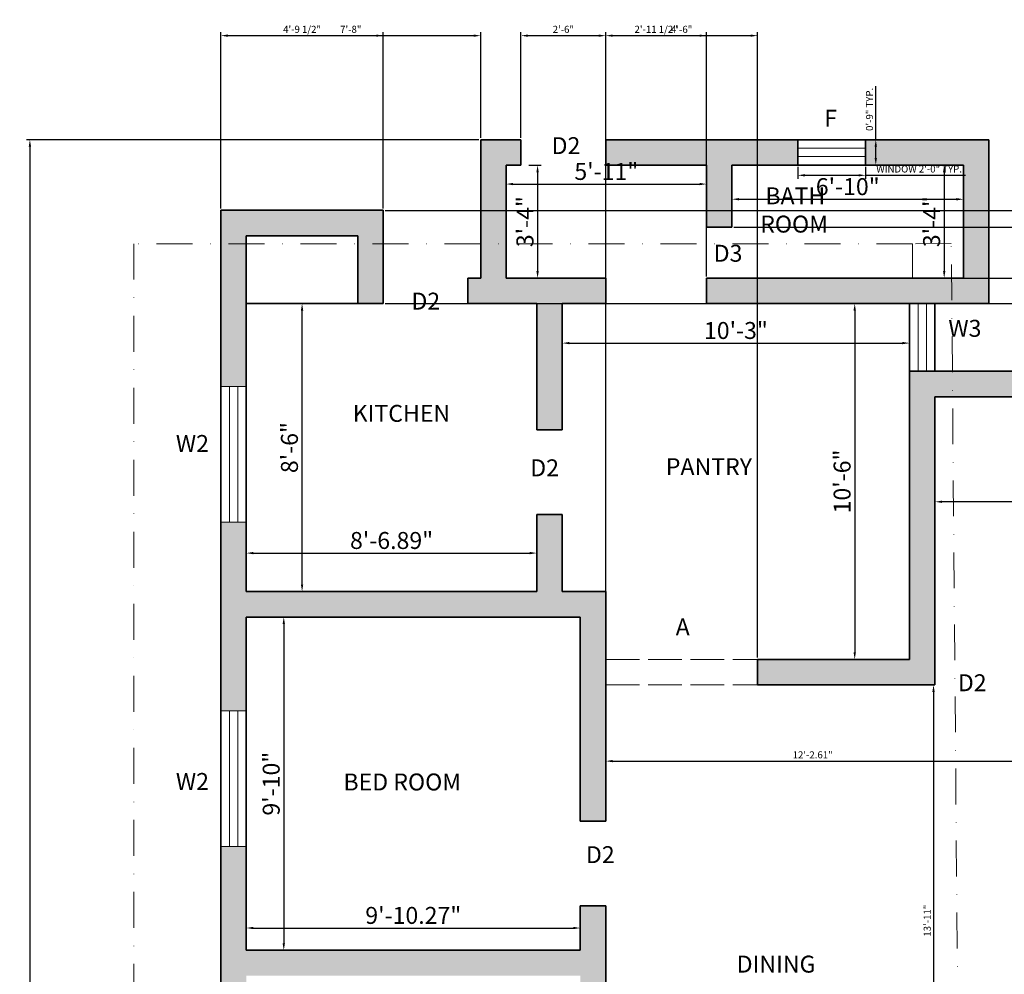
# Model space of a CAD drawing. Units: inches. Extents: x 4701 to 5398, y 2331 to 3130.
# Tile 2 of 3: x 4701 to 5050, y 2792 to 3130. Entities that reach past the tile are written whole.
import ezdxf

# ---------------------------------------------------------------- set-up
doc = ezdxf.new("R2010")
doc.units = ezdxf.units.IN
doc.linetypes.add('ACAD_ISO02W100', pattern=[15, 12, -3])
doc.linetypes.add('DASHDOT', pattern=[25.4, 12.7, -6.35, 0, -6.35])
for name, color, linetype, lineweight, true_color in [('A-ANNO-DIMS', 217, 'Continuous', 18, 0x93278f), ('A-GLAZ', 41, 'Continuous', 18, 0xf4ee51), ('A-WALL-OVHD', 41, 'ACAD_ISO02W100', 18, 0xf4ee51), ('A-WALL-PATT', 143, 'Continuous', 13, 0x7aafdf)]:
    doc.layers.add(name, color=color, linetype=linetype, lineweight=lineweight, true_color=true_color)
for name, color, linetype, lineweight in [('A-ANNO-TEXT', 7, 'Continuous', 18), ('A-AREA-IDEN', 7, 'Continuous', 25), ('A-ROOF-OVHD', 8, 'DASHDOT', 13), ('A-WALL', 7, 'Continuous', 35)]:
    doc.layers.add(name, color=color, linetype=linetype, lineweight=lineweight)
doc.styles.get("Standard").update_dxf_attribs({"font": 'arial.ttf'})
doc.dimstyles.new('ISO-25', dxfattribs={"dimtxt": 2.5, "dimasz": 2.5, "dimexe": 1.25, "dimexo": 0.625, "dimtad": 1, "dimlunit": 3, "dimtxsty": 'Standard', "dimcen": 2.5, "dimadec": 0, "dimazin": 0, "dimtfac": 1, "dimtmove": 0, "dimatfit": 3, "dimfxl": 1, "dimarcsym": 0})

# ---------------------------------------------------------------- blocks, each defined once
blk = doc.blocks.new('*D1')
at = {"layer": 'A-ANNO-DIMS', "color": 0, "lineweight": -2, "transparency": 16777216}
for p, q in [((4873.22, 3071.97), (4873.22, 3072.6)), ((4944.22, 3071.97), (4944.22, 3072.6)), ((4875.72, 3071.35), (4941.72, 3071.35))]:
    blk.add_line(p, q, dxfattribs=at)
at = {"layer": 'A-ANNO-DIMS', "color": 0, "transparency": 16777216}
for points in [[(4875.72, 3071.77), (4875.72, 3070.93), (4873.22, 3071.35)], [(4941.72, 3071.77), (4941.72, 3070.93), (4944.22, 3071.35)]]:
    blk.add_solid(points, dxfattribs=at)
at = {"layer": 'Defpoints', "color": 0, "transparency": 16777216}
for p in [(4873.22, 3071.35), (4944.22, 3071.35), (4944.22, 3071.35)]:
    blk.add_point(p, dxfattribs=at)
at = {"layer": 'A-ANNO-DIMS', "color": 0, "transparency": 16777216, "insert": (4908.72, 3075.04), "char_height": 6, "attachment_point": 5}
blk.add_mtext('5\'-11"', dxfattribs=at)
blk = doc.blocks.new('*D2')
at = {"layer": 'A-ANNO-DIMS', "color": 0, "lineweight": -2, "transparency": 16777216}
for p, q in [((4953.22, 3066.43), (4953.22, 3064.73)), ((4955.72, 3065.98), (5032.72, 3065.98)), ((5035.22, 3066.61), (5035.22, 3067.23))]:
    blk.add_line(p, q, dxfattribs=at)
at = {"layer": 'A-ANNO-DIMS', "color": 0, "transparency": 16777216}
for points in [[(4955.72, 3066.4), (4955.72, 3065.57), (4953.22, 3065.98)], [(5032.72, 3066.4), (5032.72, 3065.57), (5035.22, 3065.98)]]:
    blk.add_solid(points, dxfattribs=at)
at = {"layer": 'Defpoints', "color": 0, "transparency": 16777216}
for p in [(4953.22, 3067.05), (5035.22, 3065.98), (5035.22, 3065.98)]:
    blk.add_point(p, dxfattribs=at)
at = {"layer": 'A-ANNO-DIMS', "color": 0, "transparency": 16777216, "insert": (4994.22, 3069.67), "char_height": 6, "attachment_point": 5}
blk.add_mtext('6\'-10"', dxfattribs=at)
blk = doc.blocks.new('*D3')
at = {"layer": 'A-ANNO-DIMS', "color": 0, "lineweight": -2, "transparency": 16777216}
for p, q in [((4881.25, 3078.05), (4885.63, 3078.05)), ((4884.38, 3075.55), (4884.38, 3040.55)), ((4881.25, 3038.05), (4885.63, 3038.05))]:
    blk.add_line(p, q, dxfattribs=at)
at = {"layer": 'A-ANNO-DIMS', "color": 0, "transparency": 16777216}
for points in [[(4883.96, 3075.55), (4884.8, 3075.55), (4884.38, 3078.05)], [(4883.96, 3040.55), (4884.8, 3040.55), (4884.38, 3038.05)]]:
    blk.add_solid(points, dxfattribs=at)
at = {"layer": 'Defpoints', "color": 0, "transparency": 16777216}
for p in [(4880.63, 3078.05), (4880.63, 3038.05), (4884.38, 3038.05)]:
    blk.add_point(p, dxfattribs=at)
at = {"layer": 'A-ANNO-DIMS', "color": 0, "transparency": 16777216, "insert": (4880.69, 3058.05), "char_height": 6, "attachment_point": 5, "rotation": 90}
blk.add_mtext('3\'-4"', dxfattribs=at)
blk = doc.blocks.new('*D4')
at = {"layer": 'A-ANNO-DIMS', "color": 0, "lineweight": -2, "transparency": 16777216}
for p, q in [((5027.76, 3078.05), (5027.13, 3078.05)), ((5028.38, 3075.55), (5028.38, 3040.55)), ((5027.76, 3038.05), (5027.13, 3038.05))]:
    blk.add_line(p, q, dxfattribs=at)
at = {"layer": 'A-ANNO-DIMS', "color": 0, "transparency": 16777216}
for points in [[(5027.97, 3075.55), (5028.8, 3075.55), (5028.38, 3078.05)], [(5027.97, 3040.55), (5028.8, 3040.55), (5028.38, 3038.05)]]:
    blk.add_solid(points, dxfattribs=at)
at = {"layer": 'Defpoints', "color": 0, "transparency": 16777216}
for p in [(5028.38, 3078.05), (5028.38, 3038.05), (5028.38, 3038.05)]:
    blk.add_point(p, dxfattribs=at)
at = {"layer": 'A-ANNO-DIMS', "color": 0, "transparency": 16777216, "insert": (5024.69, 3058.05), "char_height": 6, "attachment_point": 5, "rotation": 90}
blk.add_mtext('3\'-4"', dxfattribs=at)
blk = doc.blocks.new('*D5')
at = {"layer": 'A-ANNO-DIMS', "color": 0, "lineweight": -2, "transparency": 16777216}
for p, q in [((4801.6, 3029.05), (4802.22, 3029.05)), ((4800.97, 2929.55), (4800.97, 3026.55)), ((4801.6, 2927.05), (4799.72, 2927.05))]:
    blk.add_line(p, q, dxfattribs=at)
at = {"layer": 'A-ANNO-DIMS', "color": 0, "transparency": 16777216}
for points in [[(4800.56, 3026.55), (4801.39, 3026.55), (4800.97, 3029.05)], [(4800.56, 2929.55), (4801.39, 2929.55), (4800.97, 2927.05)]]:
    blk.add_solid(points, dxfattribs=at)
at = {"layer": 'Defpoints', "color": 0, "transparency": 16777216}
for p in [(4800.97, 3029.05), (4800.97, 3029.05), (4802.22, 2927.05)]:
    blk.add_point(p, dxfattribs=at)
at = {"layer": 'A-ANNO-DIMS', "color": 0, "transparency": 16777216, "insert": (4797.28, 2978.05), "char_height": 6, "attachment_point": 5, "rotation": 90}
blk.add_mtext('8\'-6"', dxfattribs=at)
blk = doc.blocks.new('*D6')
at = {"layer": 'A-ANNO-DIMS', "color": 0, "lineweight": -2, "transparency": 16777216}
for p, q in [((4781.22, 2941.32), (4781.22, 2941.94)), ((4783.72, 2940.69), (4881.61, 2940.69)), ((4884.11, 2941.32), (4884.11, 2941.94))]:
    blk.add_line(p, q, dxfattribs=at)
at = {"layer": 'A-ANNO-DIMS', "color": 0, "transparency": 16777216}
for points in [[(4783.72, 2941.11), (4783.72, 2940.27), (4781.22, 2940.69)], [(4881.61, 2941.11), (4881.61, 2940.27), (4884.11, 2940.69)]]:
    blk.add_solid(points, dxfattribs=at)
at = {"layer": 'Defpoints', "color": 0, "transparency": 16777216}
for p in [(4781.22, 2940.69), (4884.11, 2940.69), (4884.11, 2940.69)]:
    blk.add_point(p, dxfattribs=at)
at = {"layer": 'A-ANNO-DIMS', "color": 0, "transparency": 16777216, "insert": (4832.67, 2944.38), "char_height": 6, "attachment_point": 5}
blk.add_mtext('8\'-6.89"', dxfattribs=at)
blk = doc.blocks.new('*D7')
at = {"layer": 'A-ANNO-DIMS', "color": 0, "lineweight": -2, "transparency": 16777216}
for p, q in [((4893.11, 3015.67), (4893.11, 3016.29)), ((5016.11, 3015.67), (5016.11, 3016.29)), ((4895.61, 3015.04), (5013.61, 3015.04))]:
    blk.add_line(p, q, dxfattribs=at)
at = {"layer": 'A-ANNO-DIMS', "color": 0, "transparency": 16777216}
for points in [[(4895.61, 3015.46), (4895.61, 3014.63), (4893.11, 3015.04)], [(5013.61, 3015.46), (5013.61, 3014.63), (5016.11, 3015.04)]]:
    blk.add_solid(points, dxfattribs=at)
at = {"layer": 'Defpoints', "color": 0, "transparency": 16777216}
for p in [(4893.11, 3015.04), (5016.11, 3015.04), (5016.11, 3015.04)]:
    blk.add_point(p, dxfattribs=at)
at = {"layer": 'A-ANNO-DIMS', "color": 0, "transparency": 16777216, "insert": (4954.61, 3018.73), "char_height": 6, "attachment_point": 5}
blk.add_mtext('10\'-3"', dxfattribs=at)
blk = doc.blocks.new('*D8')
at = {"layer": 'A-ANNO-DIMS', "color": 0, "lineweight": -2, "transparency": 16777216}
for p, q in [((4999.81, 3029.05), (4995.44, 3029.05)), ((4996.69, 3026.55), (4996.69, 2905.55)), ((4997.31, 2903.05), (4997.94, 2903.05))]:
    blk.add_line(p, q, dxfattribs=at)
at = {"layer": 'A-ANNO-DIMS', "color": 0, "transparency": 16777216}
for points in [[(4996.27, 3026.55), (4997.11, 3026.55), (4996.69, 3029.05)], [(4996.27, 2905.55), (4997.11, 2905.55), (4996.69, 2903.05)]]:
    blk.add_solid(points, dxfattribs=at)
at = {"layer": 'Defpoints', "color": 0, "transparency": 16777216}
for p in [(5000.44, 3029.05), (4996.69, 2903.05), (4996.69, 2903.05)]:
    blk.add_point(p, dxfattribs=at)
at = {"layer": 'A-ANNO-DIMS', "color": 0, "transparency": 16777216, "insert": (4993, 2966.05), "char_height": 6, "attachment_point": 5, "rotation": 90}
blk.add_mtext('10\'-6"', dxfattribs=at)
blk = doc.blocks.new('*D9')
at = {"layer": 'A-ANNO-DIMS', "color": 0, "lineweight": -2, "transparency": 16777216}
for p, q in [((5025.11, 2959.48), (5025.11, 2960.11)), ((5190.61, 2958.86), (5027.61, 2958.86)), ((5193.11, 2959.48), (5193.11, 2960.11))]:
    blk.add_line(p, q, dxfattribs=at)
at = {"layer": 'A-ANNO-DIMS', "color": 0, "transparency": 16777216}
for points in [[(5027.61, 2959.28), (5027.61, 2958.44), (5025.11, 2958.86)], [(5190.61, 2959.28), (5190.61, 2958.44), (5193.11, 2958.86)]]:
    blk.add_solid(points, dxfattribs=at)
at = {"layer": 'Defpoints', "color": 0, "transparency": 16777216}
for p in [(5025.11, 2958.86), (5025.11, 2958.86), (5193.11, 2958.86)]:
    blk.add_point(p, dxfattribs=at)
at = {"layer": 'A-ANNO-DIMS', "color": 0, "transparency": 16777216, "insert": (5109.11, 2962.5), "char_height": 6, "attachment_point": 5}
blk.add_mtext("14'", dxfattribs=at)
blk = doc.blocks.new('*D13')
at = {"layer": 'A-ANNO-DIMS', "color": 0, "lineweight": -2, "transparency": 16777216}
for p, q in [((4781.22, 2808.57), (4781.22, 2809.19)), ((4783.72, 2807.94), (4897, 2807.94)), ((4899.5, 2808.57), (4899.5, 2809.19))]:
    blk.add_line(p, q, dxfattribs=at)
at = {"layer": 'A-ANNO-DIMS', "color": 0, "transparency": 16777216}
for points in [[(4783.72, 2808.36), (4783.72, 2807.53), (4781.22, 2807.94)], [(4897, 2808.36), (4897, 2807.53), (4899.5, 2807.94)]]:
    blk.add_solid(points, dxfattribs=at)
at = {"layer": 'Defpoints', "color": 0, "transparency": 16777216}
for p in [(4781.22, 2807.94), (4899.5, 2807.94), (4899.5, 2807.94)]:
    blk.add_point(p, dxfattribs=at)
at = {"layer": 'A-ANNO-DIMS', "color": 0, "transparency": 16777216, "insert": (4840.36, 2811.63), "char_height": 6, "attachment_point": 5}
blk.add_mtext('9\'-10.27"', dxfattribs=at)
blk = doc.blocks.new('*D14')
at = {"layer": 'A-ANNO-DIMS', "color": 0, "lineweight": -2, "transparency": 16777216}
for p, q in [((4794.49, 2915.55), (4794.49, 2802.55)), ((4795.12, 2918.05), (4795.74, 2918.05)), ((4795.12, 2800.05), (4795.74, 2800.05))]:
    blk.add_line(p, q, dxfattribs=at)
at = {"layer": 'A-ANNO-DIMS', "color": 0, "transparency": 16777216}
for points in [[(4794.08, 2915.55), (4794.91, 2915.55), (4794.49, 2918.05)], [(4794.08, 2802.55), (4794.91, 2802.55), (4794.49, 2800.05)]]:
    blk.add_solid(points, dxfattribs=at)
at = {"layer": 'Defpoints', "color": 0, "transparency": 16777216}
for p in [(4794.49, 2918.05), (4794.49, 2800.05), (4794.49, 2800.05)]:
    blk.add_point(p, dxfattribs=at)
at = {"layer": 'A-ANNO-DIMS', "color": 0, "transparency": 16777216, "insert": (4790.81, 2859.05), "char_height": 6, "attachment_point": 5, "rotation": 90}
blk.add_mtext('9\'-10"', dxfattribs=at)
blk = doc.blocks.new('*D29')
at = {"layer": 'A-ANNO-DIMS', "color": 0, "lineweight": -2, "transparency": 16777216}
for p, q in [((4908.5, 2867.66), (4908.5, 2868.28)), ((4911, 2867.03), (5052.61, 2867.03)), ((5055.11, 2867.66), (5055.11, 2868.28))]:
    blk.add_line(p, q, dxfattribs=at)
at = {"layer": 'A-ANNO-DIMS', "color": 0, "transparency": 16777216}
for points in [[(4911, 2867.45), (4911, 2866.62), (4908.5, 2867.03)], [(5052.61, 2867.45), (5052.61, 2866.62), (5055.11, 2867.03)]]:
    blk.add_solid(points, dxfattribs=at)
at = {"layer": 'Defpoints', "color": 0, "transparency": 16777216}
for p in [(4908.5, 2867.03), (5055.11, 2867.03), (5055.11, 2867.03)]:
    blk.add_point(p, dxfattribs=at)
at = {"layer": 'A-ANNO-DIMS', "color": 0, "transparency": 16777216, "insert": (4981.8, 2868.94), "char_height": 2.5, "attachment_point": 5}
blk.add_mtext('12\'-2.61"', dxfattribs=at)
blk = doc.blocks.new('*D30')
at = {"layer": 'A-ANNO-DIMS', "color": 0, "lineweight": -2, "transparency": 16777216}
for p, q in [((5024.48, 2894.05), (5023.35, 2894.05)), ((5024.6, 2891.55), (5024.6, 2729.55)), ((5025.23, 2727.05), (5025.85, 2727.05))]:
    blk.add_line(p, q, dxfattribs=at)
at = {"layer": 'A-ANNO-DIMS', "color": 0, "transparency": 16777216}
for points in [[(5024.19, 2891.55), (5025.02, 2891.55), (5024.6, 2894.05)], [(5024.19, 2729.55), (5025.02, 2729.55), (5024.6, 2727.05)]]:
    blk.add_solid(points, dxfattribs=at)
at = {"layer": 'Defpoints', "color": 0, "transparency": 16777216}
for p in [(5025.11, 2894.05), (5024.6, 2727.05), (5024.6, 2727.05)]:
    blk.add_point(p, dxfattribs=at)
at = {"layer": 'A-ANNO-DIMS', "color": 0, "transparency": 16777216, "insert": (5022.7, 2810.55), "char_height": 2.5, "attachment_point": 5, "rotation": 90}
blk.add_mtext('13\'-11"', dxfattribs=at)
blk = doc.blocks.new('WIN-48IN')
for p, q in [((0, 48), (9, 48)), ((0, 48), (0, 0)), ((3, 48), (3, 0)), ((6, 48), (6, 0)), ((9, 0), (9, 48)), ((0, 0), (9, 0))]:
    blk.add_line(p, q)
blk = doc.blocks.new('WIN-24IN')
for p, q in [((0, 9), (0, 0)), ((24, 9), (0, 9)), ((24, 0), (24, 9)), ((24, 6), (0, 6)), ((24, 3), (0, 3)), ((0, 0), (24, 0))]:
    blk.add_line(p, q)
blk = doc.blocks.new('*D39')
at = {"layer": 'A-ANNO-DIMS', "color": 0, "lineweight": -2, "transparency": 16777216}
for p, q in [((4976.55, 3077.43), (4976.55, 3073.2)), ((5000.55, 3077.43), (5000.55, 3073.2)), ((4979.05, 3074.45), (4998.05, 3074.45)), ((5000.55, 3074.45), (5035.93, 3074.45))]:
    blk.add_line(p, q, dxfattribs=at)
at = {"layer": 'A-ANNO-DIMS', "color": 0, "transparency": 16777216}
for points in [[(4979.05, 3074.87), (4979.05, 3074.04), (4976.55, 3074.45)], [(4998.05, 3074.87), (4998.05, 3074.04), (5000.55, 3074.45)]]:
    blk.add_solid(points, dxfattribs=at)
at = {"layer": 'Defpoints', "color": 0, "transparency": 16777216}
for p in [(4976.55, 3078.05), (5000.55, 3078.05), (5000.55, 3074.45)]:
    blk.add_point(p, dxfattribs=at)
at = {"layer": 'A-ANNO-DIMS', "color": 0, "transparency": 16777216, "insert": (5019.49, 3076.37), "char_height": 2.5, "attachment_point": 5}
blk.add_mtext('WINDOW 2\'-0" TYP.', dxfattribs=at)
blk = doc.blocks.new('*D40')
at = {"layer": 'A-ANNO-DIMS', "color": 0, "lineweight": -2, "transparency": 16777216}
for p, q in [((5004.15, 3087.05), (5004.15, 3106.04)), ((5001.17, 3087.05), (5005.4, 3087.05)), ((5004.15, 3080.55), (5004.15, 3084.55)), ((5001.17, 3078.05), (5005.4, 3078.05))]:
    blk.add_line(p, q, dxfattribs=at)
at = {"layer": 'A-ANNO-DIMS', "color": 0, "transparency": 16777216}
for points in [[(5003.73, 3084.55), (5004.56, 3084.55), (5004.15, 3087.05)], [(5003.73, 3080.55), (5004.56, 3080.55), (5004.15, 3078.05)]]:
    blk.add_solid(points, dxfattribs=at)
at = {"layer": 'Defpoints', "color": 0, "transparency": 16777216}
for p in [(5000.55, 3087.05), (5004.15, 3087.05), (5000.55, 3078.05)]:
    blk.add_point(p, dxfattribs=at)
at = {"layer": 'A-ANNO-DIMS', "color": 0, "transparency": 16777216, "insert": (5002.24, 3097.8), "char_height": 2.5, "attachment_point": 5, "rotation": 90}
blk.add_mtext('0\'-9" TYP.', dxfattribs=at)
blk = doc.blocks.new('*D44')
at = {"layer": 'A-ANNO-DIMS', "color": 0, "lineweight": -2, "transparency": 16777216}
for p, q in [((4863.6, 3087.05), (4703.32, 3087.05)), ((4704.57, 3084.55), (4704.57, 2407.55)), ((4985.68, 2405.05), (4703.32, 2405.05))]:
    blk.add_line(p, q, dxfattribs=at)
at = {"layer": 'A-ANNO-DIMS', "color": 0, "transparency": 16777216}
for points in [[(4704.15, 3084.55), (4704.99, 3084.55), (4704.57, 3087.05)], [(4704.15, 2407.55), (4704.99, 2407.55), (4704.57, 2405.05)]]:
    blk.add_solid(points, dxfattribs=at)
at = {"layer": 'Defpoints', "color": 0, "transparency": 16777216}
for p in [(4864.22, 3087.05), (4704.57, 2405.05), (4986.3, 2405.05)]:
    blk.add_point(p, dxfattribs=at)
at = {"layer": 'A-ANNO-DIMS', "color": 0, "transparency": 16777216, "insert": (4702.67, 2746.05), "char_height": 2.5, "attachment_point": 5, "rotation": 90}
blk.add_mtext('56\'-10"', dxfattribs=at)
blk = doc.blocks.new('*D46')
at = {"layer": 'A-ANNO-DIMS', "color": 0, "lineweight": -2, "transparency": 16777216}
for p, q in [((4878.5, 3087.68), (4878.5, 3125.15)), ((4908.5, 3087.68), (4908.5, 3125.15)), ((4881, 3123.9), (4906, 3123.9))]:
    blk.add_line(p, q, dxfattribs=at)
at = {"layer": 'A-ANNO-DIMS', "color": 0, "transparency": 16777216}
for points in [[(4881, 3124.32), (4881, 3123.49), (4878.5, 3123.9)], [(4906, 3124.32), (4906, 3123.49), (4908.5, 3123.9)]]:
    blk.add_solid(points, dxfattribs=at)
at = {"layer": 'Defpoints', "color": 0, "transparency": 16777216}
for p in [(4908.5, 3123.9), (4878.5, 3087.05), (4908.5, 3087.05)]:
    blk.add_point(p, dxfattribs=at)
at = {"layer": 'A-ANNO-DIMS', "color": 0, "transparency": 16777216, "insert": (4893.5, 3125.81), "char_height": 2.5, "attachment_point": 5}
blk.add_mtext('2\'-6"', dxfattribs=at)
blk = doc.blocks.new('*D47')
at = {"layer": 'A-ANNO-DIMS', "color": 0, "lineweight": -2, "transparency": 16777216}
for p, q in [((4908.5, 3038.68), (4908.5, 3125.15)), ((4944.22, 3038.68), (4944.22, 3125.15)), ((4911, 3123.9), (4941.72, 3123.9))]:
    blk.add_line(p, q, dxfattribs=at)
at = {"layer": 'A-ANNO-DIMS', "color": 0, "transparency": 16777216}
for points in [[(4911, 3124.32), (4911, 3123.49), (4908.5, 3123.9)], [(4941.72, 3124.32), (4941.72, 3123.49), (4944.22, 3123.9)]]:
    blk.add_solid(points, dxfattribs=at)
at = {"layer": 'Defpoints', "color": 0, "transparency": 16777216}
for p in [(4944.22, 3123.9), (4908.5, 3038.05), (4944.22, 3038.05)]:
    blk.add_point(p, dxfattribs=at)
at = {"layer": 'A-ANNO-DIMS', "color": 0, "transparency": 16777216, "insert": (4926.36, 3125.82), "char_height": 2.5, "attachment_point": 5}
blk.add_mtext('2\'-11 1/2"', dxfattribs=at)
blk = doc.blocks.new('*D49')
at = {"layer": 'A-ANNO-DIMS', "color": 0, "lineweight": -2, "transparency": 16777216}
for p, q in [((4908.5, 2903.68), (4908.5, 3125.15)), ((4962.3, 2903.68), (4962.3, 3125.15)), ((4911, 3123.9), (4959.8, 3123.9))]:
    blk.add_line(p, q, dxfattribs=at)
at = {"layer": 'A-ANNO-DIMS', "color": 0, "transparency": 16777216}
for points in [[(4911, 3124.32), (4911, 3123.49), (4908.5, 3123.9)], [(4959.8, 3124.32), (4959.8, 3123.49), (4962.3, 3123.9)]]:
    blk.add_solid(points, dxfattribs=at)
at = {"layer": 'Defpoints', "color": 0, "transparency": 16777216}
for p in [(4962.3, 3123.9), (4908.5, 2903.05), (4962.3, 2903.05)]:
    blk.add_point(p, dxfattribs=at)
at = {"layer": 'A-ANNO-DIMS', "color": 0, "transparency": 16777216, "insert": (4935.4, 3125.81), "char_height": 2.5, "attachment_point": 5}
blk.add_mtext('4\'-6"', dxfattribs=at)
blk = doc.blocks.new('*D51')
at = {"layer": 'A-ANNO-DIMS', "color": 0, "lineweight": -2, "transparency": 16777216}
for p, q in [((4772.22, 3062.68), (4772.22, 3125.15)), ((4864.22, 3087.68), (4864.22, 3125.15)), ((4774.72, 3123.9), (4861.72, 3123.9))]:
    blk.add_line(p, q, dxfattribs=at)
at = {"layer": 'A-ANNO-DIMS', "color": 0, "transparency": 16777216}
for points in [[(4774.72, 3124.32), (4774.72, 3123.49), (4772.22, 3123.9)], [(4861.72, 3124.32), (4861.72, 3123.49), (4864.22, 3123.9)]]:
    blk.add_solid(points, dxfattribs=at)
at = {"layer": 'Defpoints', "color": 0, "transparency": 16777216}
for p in [(4864.22, 3123.9), (4864.22, 3087.05), (4772.22, 3062.05)]:
    blk.add_point(p, dxfattribs=at)
at = {"layer": 'A-ANNO-DIMS', "color": 0, "transparency": 16777216, "insert": (4818.22, 3125.81), "char_height": 2.5, "attachment_point": 5}
blk.add_mtext('7\'-8"', dxfattribs=at)
blk = doc.blocks.new('*D52')
at = {"layer": 'A-ANNO-DIMS', "color": 0, "lineweight": -2, "transparency": 16777216}
for p, q in [((4772.22, 3062.68), (4772.22, 3125.15)), ((4829.72, 3062.68), (4829.72, 3125.15)), ((4774.72, 3123.9), (4827.22, 3123.9))]:
    blk.add_line(p, q, dxfattribs=at)
at = {"layer": 'A-ANNO-DIMS', "color": 0, "transparency": 16777216}
for points in [[(4774.72, 3124.32), (4774.72, 3123.49), (4772.22, 3123.9)], [(4827.22, 3124.32), (4827.22, 3123.49), (4829.72, 3123.9)]]:
    blk.add_solid(points, dxfattribs=at)
at = {"layer": 'Defpoints', "color": 0, "transparency": 16777216}
for p in [(4829.72, 3123.9), (4772.22, 3062.05), (4829.72, 3062.05)]:
    blk.add_point(p, dxfattribs=at)
at = {"layer": 'A-ANNO-DIMS', "color": 0, "transparency": 16777216, "insert": (4800.97, 3125.82), "char_height": 2.5, "attachment_point": 5}
blk.add_mtext('4\'-9 1/2"', dxfattribs=at)
blk = doc.blocks.new('*D53')
at = {"layer": 'A-ANNO-DIMS', "color": 0, "lineweight": -2, "transparency": 16777216}
for p, q in [((4830.35, 3062.05), (5398.37, 3062.05)), ((5397.12, 3059.55), (5397.12, 3031.55)), ((4830.35, 3029.05), (5398.37, 3029.05))]:
    blk.add_line(p, q, dxfattribs=at)
at = {"layer": 'A-ANNO-DIMS', "color": 0, "transparency": 16777216}
for points in [[(5396.71, 3059.55), (5397.54, 3059.55), (5397.12, 3062.05)], [(5396.71, 3031.55), (5397.54, 3031.55), (5397.12, 3029.05)]]:
    blk.add_solid(points, dxfattribs=at)
at = {"layer": 'Defpoints', "color": 0, "transparency": 16777216}
for p in [(4829.72, 3062.05), (4829.72, 3029.05), (5397.12, 3029.05)]:
    blk.add_point(p, dxfattribs=at)
at = {"layer": 'A-ANNO-DIMS', "color": 0, "transparency": 16777216, "insert": (5395.22, 3045.55), "char_height": 2.5, "attachment_point": 5, "rotation": 90}
blk.add_mtext('2\'-9"', dxfattribs=at)
blk = doc.blocks.new('*D54')
at = {"layer": 'A-ANNO-DIMS', "color": 0, "lineweight": -2, "transparency": 16777216}
for p, q in [((4953.85, 3056.05), (5398.37, 3056.05)), ((5397.12, 3053.55), (5397.12, 3040.55)), ((4944.85, 3038.05), (5398.37, 3038.05))]:
    blk.add_line(p, q, dxfattribs=at)
at = {"layer": 'A-ANNO-DIMS', "color": 0, "transparency": 16777216}
for points in [[(5396.71, 3053.55), (5397.54, 3053.55), (5397.12, 3056.05)], [(5396.71, 3040.55), (5397.54, 3040.55), (5397.12, 3038.05)]]:
    blk.add_solid(points, dxfattribs=at)
at = {"layer": 'Defpoints', "color": 0, "transparency": 16777216}
for p in [(4953.22, 3056.05), (4944.22, 3038.05), (5397.12, 3038.05)]:
    blk.add_point(p, dxfattribs=at)
at = {"layer": 'A-ANNO-DIMS', "color": 0, "transparency": 16777216, "insert": (5395.22, 3047.05), "char_height": 2.5, "attachment_point": 5, "rotation": 90}
blk.add_mtext('1\'-6"', dxfattribs=at)

msp = doc.modelspace()

# ---------------------------------------------------------------- hatches: boundary and pattern name
at = {"layer": 'A-WALL-PATT'}
h = msp.add_hatch(color=256, dxfattribs=at)
h.dxf.hatch_style = 1
h.paths.add_polyline_path([(4829.723, 3062.054), (4820.723, 3062.054), (4772.223, 3062.054), (4772.223, 3050.208), (4781.223, 3050.208), (4781.223, 3053.054), (4820.723, 3053.054), (4820.723, 3050.208), (4829.723, 3050.208)])
h.paths.add_polyline_path([(4781.223, 3050.208), (4772.223, 3050.208), (4772.223, 3029.054), (4772.223, 2999.675), (4781.223, 2999.675), (4781.223, 3029.054)])
h.paths.add_polyline_path([(4781.223, 2918.054), (4864.223, 2918.054), (4899.497, 2918.054), (4899.497, 2845.832), (4908.497, 2845.832), (4908.497, 2918.054), (4908.497, 2927.054), (4893.11, 2927.054), (4893.11, 2954.328), (4884.11, 2954.328), (4884.11, 2927.054), (4864.223, 2927.054), (4781.223, 2927.054), (4781.223, 2951.675), (4772.223, 2951.675), (4772.223, 2918.054), (4772.223, 2884.79), (4781.223, 2884.79)])
h.paths.add_polyline_path([(4893.11, 3029.054), (4908.497, 3029.054), (4908.497, 3038.054), (4873.223, 3038.054), (4873.223, 3050.208), (4864.223, 3050.208), (4864.223, 3038.054), (4859.723, 3038.054), (4859.723, 3029.054), (4884.11, 3029.054), (4884.11, 2984.328), (4893.11, 2984.328)])
h.paths.add_polyline_path([(4873.223, 3078.054), (4878.497, 3078.054), (4878.497, 3087.054), (4864.223, 3087.054), (4864.223, 3050.208), (4873.223, 3050.208)])
h.paths.add_polyline_path([(4976.546, 3087.054), (4908.497, 3087.054), (4908.497, 3078.054), (4944.223, 3078.054), (4944.223, 3056.054), (4953.223, 3056.054), (4953.223, 3078.054), (4976.546, 3078.054)])
h.paths.add_polyline_path([(5044.223, 3087.054), (5000.546, 3087.054), (5000.546, 3078.054), (5035.223, 3078.054), (5035.223, 3038.054), (5044.223, 3038.054)])
h.paths.add_polyline_path([(5030.994, 3038.054), (5017.16, 3038.054), (4944.223, 3038.054), (4944.223, 3029.054), (5031.069, 3029.054)])
h.paths.add_polyline_path([(5044.223, 3038.054), (5035.223, 3038.054), (5030.994, 3038.054), (5031.069, 3029.054), (5044.223, 3029.054)])
h.paths.add_polyline_path([(5202.11, 3005.054), (5193.11, 3005.054), (5031.27, 3005.054), (5031.345, 2996.054), (5193.11, 2996.054), (5193.11, 2978.066), (5202.11, 2978.066), (5202.11, 2996.054)])
h.paths.add_polyline_path([(5031.27, 3005.054), (5025.11, 3005.054), (5016.11, 3005.054), (5016.11, 2903.054), (4962.304, 2903.054), (4962.304, 2894.054), (5025.11, 2894.054), (5025.11, 2996.054), (5031.345, 2996.054)])
h.paths.add_polyline_path([(5278.045, 2894.054), (5202.11, 2894.054), (5202.11, 2900.054), (5202.11, 2918.066), (5193.11, 2918.066), (5193.11, 2900.054), (5193.11, 2894.054), (5055.11, 2894.054), (5055.11, 2840.014), (5055.11, 2813.236), (5064.11, 2813.236), (5064.11, 2840.014), (5064.11, 2885.054), (5268.987, 2885.054)])
h.paths.add_polyline_path([(5301.11, 2894.054), (5278.045, 2894.054), (5268.987, 2885.054), (5292.11, 2885.054), (5292.11, 2855.934), (5301.11, 2855.934), (5301.11, 2885.054)])
h.paths.add_polyline_path([(5301.11, 2795.934), (5292.11, 2795.934), (5292.11, 2753.054), (5193.11, 2753.054), (5160.11, 2753.054), (5160.11, 2735.907), (5168.378, 2726.63), (5169.11, 2726.63), (5169.11, 2744.054), (5292.11, 2744.054), (5292.11, 2636.054), (5283.654, 2636.054), (5283.654, 2627.054), (5301.11, 2627.054)])
h.paths.add_polyline_path([(5160.11, 2735.907), (5160.11, 2726.63), (5168.378, 2726.63)], flags=17)
h.paths.add_polyline_path([(5064.11, 2746.827), (5055.11, 2746.827), (5055.11, 2727.054), (5033.595, 2727.054), (5033.671, 2718.054), (5055.11, 2718.054), (5055.11, 2627.054), (5055.11, 2546.054), (5035.539, 2546.054), (5035.539, 2537.054), (5064.11, 2537.054), (5064.11, 2627.054), (5074.819, 2627.054), (5074.819, 2636.054), (5064.11, 2636.054)])
h.paths.add_polyline_path([(5178.11, 2636.054), (5169.11, 2636.054), (5169.11, 2696.63), (5160.11, 2696.63), (5160.11, 2636.054), (5116.819, 2636.054), (5116.819, 2627.054), (5178.11, 2627.054)])
h.paths.add_polyline_path([(5235.654, 2636.054), (5220.11, 2636.054), (5220.11, 2627.054), (5235.654, 2627.054)], flags=17)
h.paths.add_polyline_path([(5033.595, 2727.054), (4994.096, 2727.054), (4994.096, 2718.054), (5033.671, 2718.054)])
h.paths.add_polyline_path([(4964.096, 2727.054), (4947.11, 2727.054), (4947.11, 2546.054), (4908.497, 2546.054), (4908.497, 2554.169), (4899.497, 2554.169), (4899.497, 2546.054), (4869.656, 2546.054), (4869.656, 2537.054), (4908.497, 2537.054), (4975.539, 2537.054), (4975.539, 2546.054), (4956.11, 2546.054), (4956.11, 2718.054), (4964.096, 2718.054)])
h.paths.add_polyline_path([(4827.656, 2546.054), (4781.223, 2546.054), (4781.223, 2577.475), (4772.223, 2577.475), (4772.223, 2537.054), (4827.656, 2537.054)])
h.paths.add_polyline_path([(4781.223, 2664.054), (4899.497, 2664.054), (4899.497, 2584.169), (4908.497, 2584.169), (4908.497, 2683.844), (4899.497, 2683.844), (4899.497, 2673.054), (4781.223, 2673.054), (4781.223, 2710.334), (4772.223, 2710.334), (4772.223, 2625.475), (4781.223, 2625.475)])
h.paths.add_polyline_path([(4908.497, 2815.832), (4899.497, 2815.832), (4899.497, 2800.054), (4864.223, 2800.054), (4781.223, 2800.054), (4781.223, 2836.79), (4772.223, 2836.79), (4772.223, 2758.334), (4781.223, 2758.334), (4781.223, 2791.054), (4899.497, 2791.054), (4899.497, 2713.844), (4908.497, 2713.844)])
h = msp.add_hatch(color=256, dxfattribs=at)
h.dxf.hatch_style = 1
h.paths.add_polyline_path([(4829.723, 3050.208), (4820.723, 3050.208), (4820.723, 3029.054), (4829.723, 3029.054), (4829.723, 3038.054)])

# ---------------------------------------------------------------- linework, layer by layer
at = {"layer": 'A-ROOF-OVHD'}
for p, q in [((5017.16, 3050.208), (4741.42, 3050.208)), ((4741.42, 3050.208), (4741.42, 2494.747)), ((5030.892, 3050.253), (5017.16, 3050.208)), ((5017.16, 3038.054), (5017.16, 3050.208)), ((5017.16, 3050.208), (5017.16, 3050.208)), ((5035.539, 2494.747), (5030.892, 3050.253)), ((5235.648, 3038.054), (5017.16, 3038.054))]:
    msp.add_line(p, q, dxfattribs=at)
at = {"layer": 'A-WALL'}
for p, q in [((4864.223, 3087.054), (4878.497, 3087.054)), ((4864.223, 3038.054), (4864.223, 3087.054)), ((4878.497, 3087.054), (4878.497, 3078.054)), ((4908.497, 3087.054), (4908.497, 3078.054)), ((4908.497, 3087.054), (5044.223, 3087.054)), ((4976.546, 3087.054), (4976.546, 3078.054)), ((5000.546, 3087.054), (5000.546, 3078.054)), ((5044.223, 3087.054), (5044.223, 3029.054)), ((4873.223, 3078.054), (4878.497, 3078.054)), ((4873.223, 3038.054), (4873.223, 3078.054)), ((4908.497, 3078.054), (4944.223, 3078.054)), ((4944.223, 3056.054), (4944.223, 3078.054)), ((4953.223, 3056.054), (4953.223, 3078.054)), ((4953.223, 3078.054), (5035.223, 3078.054)), ((5035.223, 3078.054), (5035.223, 3038.054)), ((4772.223, 3029.054), (4772.223, 3062.054)), ((4820.723, 3062.054), (4772.223, 3062.054)), ((4829.723, 3062.054), (4820.723, 3062.054)), ((4829.723, 3038.054), (4829.723, 3062.054)), ((4953.223, 3056.054), (4944.223, 3056.054)), ((4781.223, 3029.054), (4781.223, 3053.054)), ((4820.723, 3053.054), (4781.223, 3053.054)), ((4820.723, 3029.054), (4820.723, 3053.054)), ((4829.723, 3038.054), (4829.723, 3029.054)), ((4864.223, 3038.054), (4859.723, 3038.054)), ((4859.723, 3038.054), (4859.723, 3029.054)), ((4908.497, 3038.054), (4873.223, 3038.054)), ((4908.497, 3038.054), (4908.497, 3029.054)), ((5035.223, 3038.054), (4944.223, 3038.054)), ((4944.223, 3038.054), (4944.223, 3029.054)), ((4772.223, 3029.054), (4772.223, 2918.054)), ((4781.223, 3029.054), (4781.223, 2927.054)), ((4781.223, 3029.054), (4820.723, 3029.054)), ((4829.723, 3029.054), (4820.723, 3029.054)), ((4859.723, 3029.054), (4864.223, 3029.054)), ((4859.723, 3029.054), (4884.11, 3029.054)), ((4884.11, 3029.054), (4864.223, 3029.054)), ((4884.11, 3029.054), (4884.11, 2984.328)), ((4908.497, 3029.054), (4893.11, 3029.054)), ((4908.497, 3029.054), (4893.11, 3029.054)), ((4893.11, 3029.054), (4893.11, 2984.328)), ((4893.11, 3029.054), (4908.497, 3029.054)), ((5044.223, 3029.054), (4944.223, 3029.054)), ((5016.11, 3029.054), (5016.11, 2903.054)), ((5025.11, 3029.054), (5025.11, 3005.054)), ((5025.11, 3005.054), (5016.11, 3005.054)), ((5025.11, 3005.054), (5193.11, 3005.054)), ((5025.11, 2996.054), (5025.11, 2894.054)), ((5025.11, 2996.054), (5193.11, 2996.054)), ((4893.11, 2984.328), (4884.11, 2984.328)), ((4893.11, 2954.328), (4884.11, 2954.328)), ((4884.11, 2954.328), (4884.11, 2927.054)), ((4893.11, 2954.328), (4893.11, 2927.054)), ((4781.223, 2927.054), (4864.223, 2927.054)), ((4884.11, 2927.054), (4864.223, 2927.054)), ((4908.497, 2927.054), (4893.11, 2927.054)), ((4908.497, 2927.054), (4908.497, 2875.22)), ((4772.223, 2918.054), (4772.223, 2537.054)), ((4781.223, 2918.054), (4864.223, 2918.054)), ((4781.223, 2918.054), (4781.223, 2800.054)), ((4899.497, 2918.054), (4864.223, 2918.054)), ((4899.497, 2918.054), (4899.497, 2845.832)), ((4908.497, 2918.054), (4908.497, 2845.832)), ((5016.11, 2903.054), (4962.304, 2903.054)), ((5016.11, 2903.054), (4962.304, 2903.054)), ((4962.304, 2903.054), (4962.304, 2894.054)), ((5025.11, 2894.054), (4962.304, 2894.054)), ((4899.497, 2845.832), (4908.497, 2845.832)), ((4899.497, 2815.832), (4908.497, 2815.832)), ((4899.497, 2815.832), (4899.497, 2800.054)), ((4908.497, 2815.832), (4908.497, 2713.844)), ((4781.223, 2800.054), (4864.223, 2800.054)), ((4899.497, 2800.054), (4864.223, 2800.054))]:
    msp.add_line(p, q, dxfattribs=at)
at = {"layer": 'A-WALL-OVHD'}
for p, q in [((4908.497, 2903.054), (4962.304, 2903.054)), ((4908.497, 2894.054), (4962.304, 2894.054))]:
    msp.add_line(p, q, dxfattribs=at)

# ---------------------------------------------------------------- block references
at = {"layer": 'A-GLAZ'}
for name, p in [('WIN-24IN', (4976.546, 3078.054)), ('WIN-48IN', (4772.223, 2951.675)), ('WIN-48IN', (4772.223, 2836.791))]:
    msp.add_blockref(name, p, dxfattribs=at)
at = {"layer": 'A-GLAZ', "rotation": 90.00000000000261}
msp.add_blockref('WIN-24IN', (5025.11, 3005.054), dxfattribs=at)

# ---------------------------------------------------------------- texts
at = {"layer": 'A-ANNO-TEXT', "char_height": 6, "attachment_point": 1}
for s, insert in [('F', (4985.916, 3097.658)), ('D2', (4889.35, 3087.955)), ('D3', (4946.749, 3049.851)), ('D2', (4839.694, 3032.903)), ('W3', (5029.842, 3023.277)), ('W2', (4756.272, 2982.503)), ('D2', (4881.788, 2973.878)), ('A', (4933.292, 2917.535)), ('D2', (5033.215, 2897.778)), ('W2', (4756.272, 2862.833)), ('D2', (4901.504, 2836.913))]:
    msp.add_mtext_dynamic_manual_height_columns(s, width=53.21859, gutter_width=12.5, heights=[0], dxfattribs=dict(at, insert=insert))
at = {"layer": 'A-AREA-IDEN', "char_height": 6, "attachment_point": 1}
for s, insert in [(' BATH      ROOM', (4963.218, 3070.181)), (' KITCHEN', (4817.071, 2993.167)), ('PANTRY', (4929.794, 2974.295)), (' BED ROOM', (4813.785, 2862.65)), (' DINING', (4953.059, 2798.161))]:
    msp.add_mtext_dynamic_manual_height_columns(s, width=53.21859, gutter_width=12.5, heights=[0], dxfattribs=dict(at, insert=insert))

# ---------------------------------------------------------------- dimensions: what is measured, and where the dimension line sits
at = {"layer": 'A-ANNO-DIMS'}
for base, p1, p2, override, picture, middle in [((4829.723, 3123.904), (4772.223, 3062.054), (4829.723, 3062.054), {"dimdec": 1, "dimlfac": 1, "dimrnd": 0, "dimzin": 1, "dimdsep": 46, "dimlunit": 4, "dimfrac": 2}, '*D52', (4800.973, 3125.822)), ((4944.223, 3123.904), (4908.497, 3038.054), (4944.223, 3038.054), {"dimdec": 1, "dimlfac": 1, "dimrnd": 0, "dimzin": 1, "dimdsep": 46, "dimlunit": 4, "dimfrac": 2}, '*D47', (4926.36, 3125.822)), ((4864.223, 3123.904), (4772.223, 3062.054), (4864.223, 3087.054), {"dimdec": 1, "dimlfac": 1, "dimrnd": 0, "dimzin": 1, "dimdsep": 46, "dimlunit": 4, "dimfrac": 2}, '*D51', (4818.223, 3125.806)), ((4908.497, 3123.904), (4878.497, 3087.054), (4908.497, 3087.054), {"dimdec": 1, "dimlfac": 1, "dimrnd": 0, "dimzin": 1, "dimdsep": 46, "dimlunit": 4, "dimfrac": 2}, '*D46', (4893.497, 3125.806)), ((4962.304, 3123.904), (4908.497, 2903.054), (4962.304, 2903.054), {"dimdec": 1, "dimlfac": 1, "dimrnd": 0, "dimzin": 1, "dimdsep": 46, "dimlunit": 4, "dimfrac": 2}, '*D49', (4935.4, 3125.806)), ((5016.11, 3015.044), (4893.11, 3015.044), (5016.11, 3015.044), {"dimtxt": 6, "dimclrd": 0, "dimclre": 0, "dimclrt": 0}, '*D7', (4954.61, 3018.735)), ((5025.11, 2958.859), (5193.11, 2958.859), (5025.11, 2958.859), {"dimtxt": 6, "dimclrd": 0, "dimclre": 0, "dimclrt": 0}, '*D9', (5109.11, 2962.496)), ((4884.11, 2940.691), (4781.223, 2940.691), (4884.11, 2940.691), {"dimtxt": 6, "dimclrd": 0, "dimclre": 0, "dimclrt": 0}, '*D6', (4832.666, 2944.38)), ((5055.11, 2867.034), (4908.497, 2867.034), (5055.11, 2867.034), {"dimclrd": 0, "dimclre": 0, "dimclrt": 0}, '*D29', (4981.804, 2868.936)), ((4899.497, 2807.943), (4781.223, 2807.943), (4899.497, 2807.943), {"dimtxt": 6, "dimclrd": 0, "dimclre": 0, "dimclrt": 0}, '*D13', (4840.36, 2811.632))]:
    dim = msp.add_linear_dim(base=base, p1=p1, p2=p2, dimstyle='ISO-25', override=override, dxfattribs=at)
    dim.commit()
    dim.dimension.update_dxf_attribs({"geometry": picture, "text_midpoint": middle})
dim = msp.add_linear_dim(base=(5004.146, 3087.054), p1=(5000.546, 3078.054), p2=(5000.546, 3087.054), angle=90, text='<> TYP.', dimstyle='ISO-25', override={"dimdec": 1, "dimlfac": 1, "dimrnd": 0, "dimzin": 1, "dimdsep": 46, "dimlunit": 4, "dimfrac": 2}, dxfattribs=at)
dim.commit()
dim.dimension.update_dxf_attribs({"geometry": '*D40', "text_midpoint": (5002.245, 3097.799)})
for base, p1, p2, override, picture, middle in [((4704.57, 2405.054), (4864.223, 3087.054), (4986.304, 2405.054), {"dimdec": 1, "dimlfac": 1, "dimrnd": 0, "dimzin": 1, "dimdsep": 46, "dimlunit": 4, "dimfrac": 2}, '*D44', (4702.669, 2746.054)), ((5397.124, 3029.054), (4829.723, 3062.054), (4829.723, 3029.054), {"dimdec": 1, "dimlfac": 1, "dimrnd": 0, "dimzin": 1, "dimdsep": 46, "dimlunit": 4, "dimfrac": 2}, '*D53', (5395.223, 3045.554)), ((5397.124, 3038.054), (4953.223, 3056.054), (4944.223, 3038.054), {"dimdec": 1, "dimlfac": 1, "dimrnd": 0, "dimzin": 1, "dimdsep": 46, "dimlunit": 4, "dimfrac": 2}, '*D54', (5395.223, 3047.054)), ((4800.973, 3029.054), (4802.223, 2927.054), (4800.973, 3029.054), {"dimtxt": 6, "dimclrd": 0, "dimclre": 0, "dimclrt": 0}, '*D5', (4797.284, 2978.054)), ((4996.688, 2903.054), (5000.438, 3029.054), (4996.688, 2903.054), {"dimtxt": 6, "dimclrd": 0, "dimclre": 0, "dimclrt": 0}, '*D8', (4993, 2966.054)), ((4794.494, 2800.054), (4794.494, 2918.054), (4794.494, 2800.054), {"dimtxt": 6, "dimclrd": 0, "dimclre": 0, "dimclrt": 0}, '*D14', (4790.806, 2859.054)), ((5024.603, 2727.054), (5025.11, 2894.054), (5024.603, 2727.054), {"dimclrd": 0, "dimclre": 0, "dimclrt": 0}, '*D30', (5022.701, 2810.554))]:
    dim = msp.add_linear_dim(base=base, p1=p1, p2=p2, angle=90, dimstyle='ISO-25', override=override, dxfattribs=at)
    dim.commit()
    dim.dimension.update_dxf_attribs({"geometry": picture, "text_midpoint": middle})
for base, p1, p2, picture, middle in [((4944.223, 3071.349), (4873.223, 3071.349), (4944.223, 3071.349), '*D1', (4908.723, 3071.349)), ((5035.223, 3065.984), (4953.223, 3067.054), (5035.223, 3065.984), '*D2', (4994.223, 3065.984))]:
    dim = msp.add_linear_dim(base=base, p1=p1, p2=p2, dimstyle='ISO-25', override={"dimtxt": 6, "dimclrd": 0, "dimclre": 0, "dimclrt": 0}, dxfattribs=at)
    dim.commit()
    dim.dimension.update_dxf_attribs({"geometry": picture, "text_midpoint": middle, "dimtype": 160})
dim = msp.add_linear_dim(base=(5000.546, 3074.454), p1=(4976.546, 3078.054), p2=(5000.546, 3078.054), text='WINDOW <> TYP.', dimstyle='ISO-25', override={"dimdec": 1, "dimlfac": 1, "dimrnd": 0, "dimzin": 1, "dimdsep": 46, "dimlunit": 4, "dimfrac": 2}, dxfattribs=at)
dim.commit()
dim.dimension.update_dxf_attribs({"geometry": '*D39', "text_midpoint": (5019.489, 3076.373)})
for base, p1, p2, picture, middle in [((4884.38, 3038.054), (4880.63, 3078.054), (4880.63, 3038.054), '*D3', (4884.38, 3058.054)), ((5028.382, 3038.054), (5028.382, 3078.054), (5028.382, 3038.054), '*D4', (5028.382, 3058.054))]:
    dim = msp.add_linear_dim(base=base, p1=p1, p2=p2, angle=90, dimstyle='ISO-25', override={"dimtxt": 6, "dimclrd": 0, "dimclre": 0, "dimclrt": 0}, dxfattribs=at)
    dim.commit()
    dim.dimension.update_dxf_attribs({"geometry": picture, "text_midpoint": middle, "dimtype": 160})

doc.saveas('drawing.dxf')
